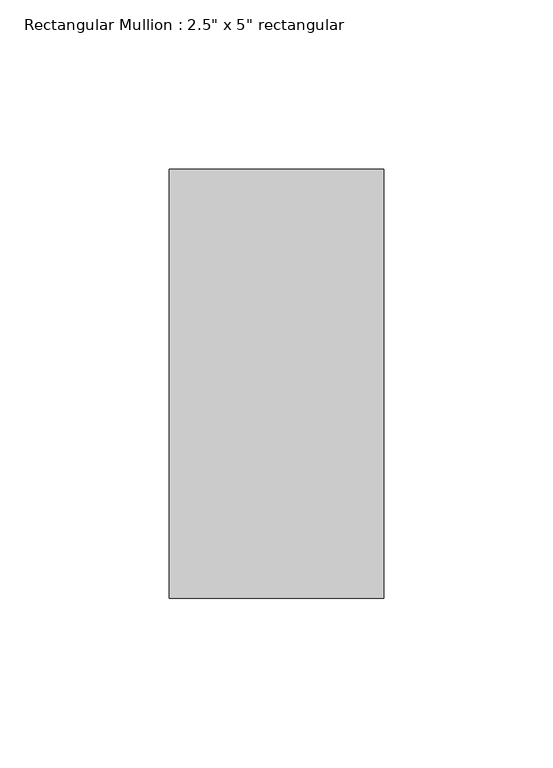
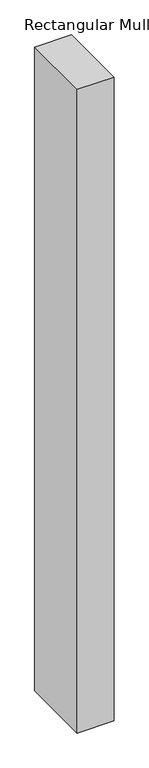
"""IFC4 building model written with IfcOpenShell, lengths in millimetres: member geometry."""

from ifc_helpers import new_model, si_unit, frame, origin, place, context, project, spatial, polyline, outline, extrude, source, transform, mapped, element, save


def member_fb497cbf(model_context):
    return source(origin(), model_context, "Body", "SweptSolid", [
        extrude(outline(polyline([(0.0, 63.5), (0.0, -63.5), (-63.5, -63.5), (-63.5, 63.5), (0.0, 63.5)])), frame((0.0, 0.0, -1174.75), z_axis=(0.0, 0.0, 1.0), x_axis=(1.0, 0.0, 0.0)), (0.0, 0.0, 1.0), 1174.75),
    ])


if __name__ == "__main__":
    model = new_model("IFC4")
    model_context = context("Model", 3, world=origin())
    ifc_project = project(units=[si_unit("LENGTHUNIT", "METRE", prefix="MILLI")], contexts=[model_context])
    site = spatial("IfcSite", under=ifc_project)
    building = spatial("IfcBuilding", under=site)
    placement = place(None, origin())
    member_shape = member_fb497cbf(model_context)
    element("IfcMember", 1, ObjectType="Rectangular Mullion : 2.5\" x 5\" rectangular", at=placement, inside=building, context=model_context, shape_type="MappedRepresentation", body=[
        mapped(member_shape, transform((0.0, 0.0, 0.0), x_axis=(1.0, 0.0, 0.0), y_axis=(0.0, 1.0, 0.0), z_axis=(0.0, 0.0, 1.0))),
    ])
    save(model, "model.ifc")

# Revit data of these elements
# Type "Rectangular Mullion : 2.5\" x 5\" rectangular"
#   built-in parameter 1007304 = 0.416667 (stored number, unit not read)
#   built-in parameter 1007301 = 0.104167 (stored number, unit not read)
#   built-in parameter 1007300 = 0.104167 (stored number, unit not read)
# Element 1 (IfcMember, "Rectangular Mullion : 2.5\" x 5\" rectangular")
#   Materials on its faces: "Aluminum"
# Materials
#   "Aluminum": class "Metal", colour RGB 247 247 247, transparency 0, Description = "Aluminum 6061", Cost = 0
